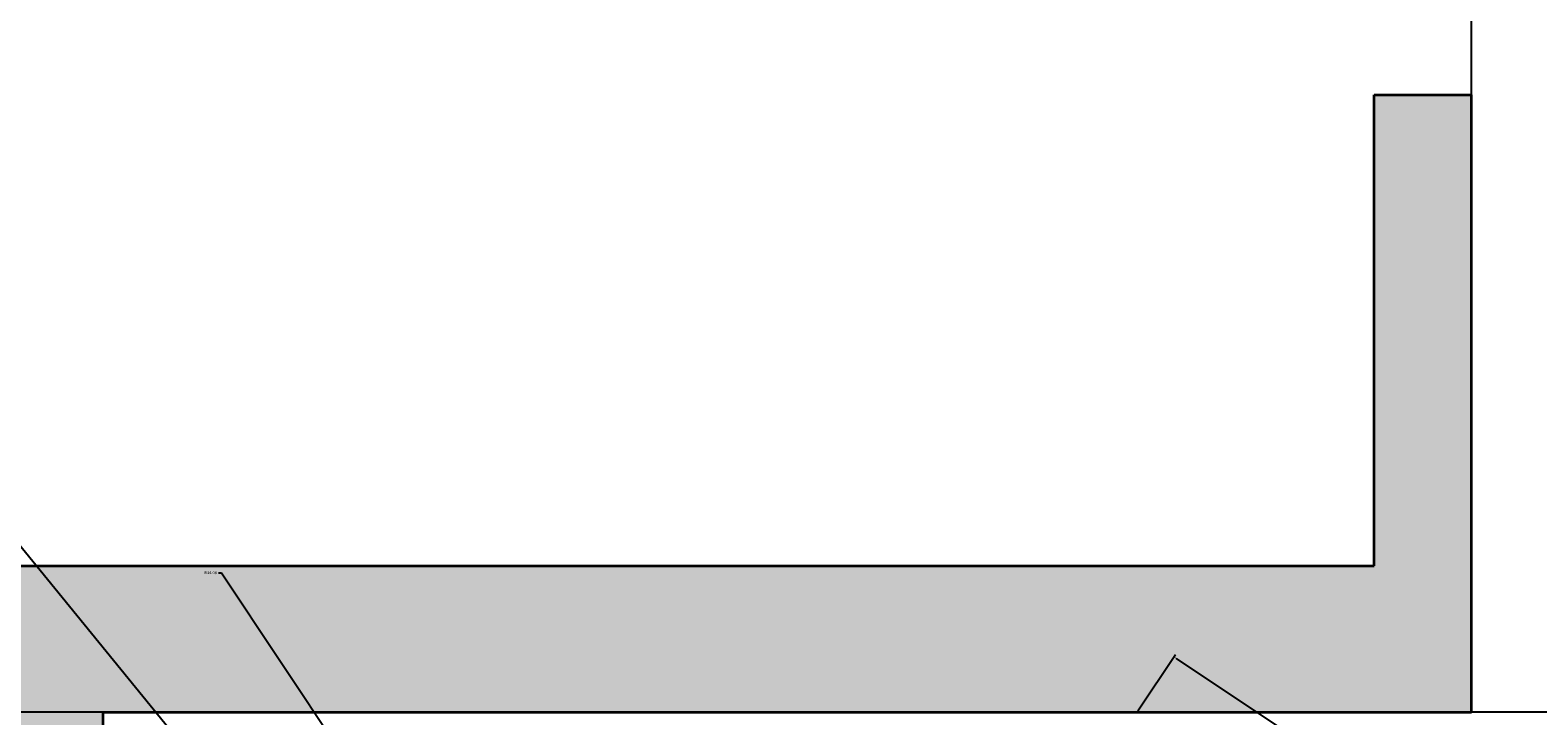
# Model space of a CAD drawing. Units: inches. Extents: x 2549 to 3108, y 1683 to 2362.
# Tile 5 of 30: x 2877 to 2970, y 1936 to 1979. Entities that reach past the tile are written whole.
import ezdxf

# ---------------------------------------------------------------- set-up
doc = ezdxf.new("R2010")
doc.units = ezdxf.units.IN
for name, color, linetype, lineweight in [('A-ANNO-DIMS', 2, 'Continuous', 18), ('A-WALL', 7, 'Continuous', 35), ('A-WALL-PATT', 89, 'Continuous', 13)]:
    doc.layers.add(name, color=color, linetype=linetype, lineweight=lineweight)
doc.layers.add('C-PKNG-VEHI-PATT', color=251, linetype='Continuous', lineweight=13, true_color=0x636466)
doc.layers.add('C-PVMT-PATT', color=9, linetype='Continuous', lineweight=13, true_color=0xc7c8ca)
doc.styles.get("Standard").update_dxf_attribs({"font": 'arial.ttf'})
doc.dimstyles.get("Standard").update_dxf_attribs({"dimtxt": 0.18, "dimasz": 0.18, "dimexe": 0.18, "dimexo": 0.0625, "dimgap": 0.09, "dimtad": 0, "dimtih": 1, "dimtoh": 1, "dimdec": 4, "dimzin": 0, "dimdsep": 46, "dimtxsty": 'Standard', "dimcen": 0.09, "dimadec": 0, "dimazin": 0, "dimtfac": 1, "dimtdec": 4, "dimtofl": 0, "dimtmove": 0, "dimatfit": 3, "dimfxl": 1, "dimtolj": 1, "dimtzin": 0, "dimarcsym": 0})

# ---------------------------------------------------------------- blocks, each defined once
blk = doc.blocks.new('*D19')
at = {"layer": 'A-ANNO-DIMS', "color": 0, "lineweight": -2, "transparency": 16777216}
for p, q in [((2945.38949374051, 1936.610352371541), (2947.701205969521, 1940.077920715058)), ((2947.751128987182, 1939.828305626757), (2957.49632815957, 1933.331506178498)), ((2967.782816554333, 1926.473847248657), (2958.037617381944, 1932.970646696915)), ((2965.720719413623, 1923.0562019228), (2968.032431642634, 1926.523770266317))]:
    blk.add_line(p, q, dxfattribs=at)
at = {"layer": 'A-ANNO-DIMS', "color": 0, "transparency": 16777216}
for points in [[(2947.767769993069, 1939.853267135587), (2947.734487981295, 1939.803344117927), (2947.6013599342, 1939.928151662078)], [(2967.799457560219, 1926.498808757487), (2967.766175548446, 1926.448885739827), (2967.932585607313, 1926.374001213336)]]:
    blk.add_solid(points, dxfattribs=at)
at = {"layer": 'Defpoints', "color": 0, "transparency": 16777216}
for p in [(2947.6013599342, 1939.928151662078), (2945.354824978246, 1936.558349228145), (2965.686050651358, 1923.004198779404)]:
    blk.add_point(p, dxfattribs=at)
at = {"layer": 'A-ANNO-DIMS', "color": 0, "transparency": 16777216, "insert": (2957.766972770757, 1933.151076437707), "char_height": 0.18, "attachment_point": 5}
blk.add_mtext('\\A1;24 TYP.', dxfattribs=at)
blk = doc.blocks.new('*D46')
at = {"layer": 'A-ANNO-DIMS', "color": 0, "lineweight": -2, "transparency": 16777216}
for p, q in [((2812.642666, 2140.461244), (2812.642666, 1683.443744)), ((3034.642666, 2134.461244), (3034.642666, 1683.443744)), ((2812.822666, 1683.623744), (2923.35320488131, 1683.623744)), ((3034.462666, 1683.623744), (2923.932127118691, 1683.623744))]:
    blk.add_line(p, q, dxfattribs=at)
at = {"layer": 'A-ANNO-DIMS', "color": 0, "transparency": 16777216}
for points in [[(2812.822666, 1683.653744), (2812.822666, 1683.593744), (2812.642666, 1683.623744)], [(3034.462666, 1683.653744), (3034.462666, 1683.593744), (3034.642666, 1683.623744)]]:
    blk.add_solid(points, dxfattribs=at)
at = {"layer": 'Defpoints', "color": 0, "transparency": 16777216}
for p in [(2812.642666, 2140.523744), (3034.642666, 2134.523744), (3034.642666, 1683.623744)]:
    blk.add_point(p, dxfattribs=at)
at = {"layer": 'A-ANNO-DIMS', "color": 0, "transparency": 16777216, "insert": (2923.642666000001, 1683.623744), "char_height": 0.18, "attachment_point": 5}
blk.add_mtext('\\A1;222', dxfattribs=at)
blk = doc.blocks.new('*D56')
at = {"layer": 'A-ANNO-DIMS', "color": 0, "lineweight": -2, "transparency": 16777216}
for p, q in [((3043.580166000001, 1936.523744000001), (2549.424763000002, 1936.523744000001)), ((2549.604763000002, 1936.343744000001), (2549.604763000002, 1911.205647137791)), ((2549.604763000002, 1885.703744000001), (2549.604763000002, 1910.841840862211)), ((3043.580166000001, 1885.523744000001), (2549.424763000002, 1885.523744000001))]:
    blk.add_line(p, q, dxfattribs=at)
at = {"layer": 'A-ANNO-DIMS', "color": 0, "transparency": 16777216}
for points in [[(2549.574763000002, 1936.343744000001), (2549.634763000002, 1936.343744000001), (2549.604763000002, 1936.523744000001)], [(2549.574763000002, 1885.703744000001), (2549.634763000002, 1885.703744000001), (2549.604763000002, 1885.523744000001)]]:
    blk.add_solid(points, dxfattribs=at)
at = {"layer": 'Defpoints', "color": 0, "transparency": 16777216}
for p in [(2549.604763000002, 1936.523744000001), (3043.642666000001, 1936.523744000001), (3043.642666000001, 1885.523744000001)]:
    blk.add_point(p, dxfattribs=at)
at = {"layer": 'A-ANNO-DIMS', "color": 0, "transparency": 16777216, "insert": (2549.604763000002, 1911.023743999999), "char_height": 0.18, "attachment_point": 5}
blk.add_mtext('\\A1;51', dxfattribs=at)
blk = doc.blocks.new('*D57')
at = {"layer": 'A-ANNO-DIMS', "color": 0, "lineweight": -2, "transparency": 16777216}
for p, q in [((2965.93514, 1936.586244), (2965.93514, 2362.322518)), ((2966.11514, 2362.142518), (2999.912081717599, 2362.142518)), ((3034.462666, 2362.142518), (3000.665724282401, 2362.142518)), ((3034.642666, 1936.586244), (3034.642666, 2362.322518))]:
    blk.add_line(p, q, dxfattribs=at)
at = {"layer": 'A-ANNO-DIMS', "color": 0, "transparency": 16777216}
for points in [[(2966.11514, 2362.172518), (2966.11514, 2362.112518), (2965.93514, 2362.142518)], [(3034.462666, 2362.172518), (3034.462666, 2362.112518), (3034.642666, 2362.142518)]]:
    blk.add_solid(points, dxfattribs=at)
at = {"layer": 'Defpoints', "color": 0, "transparency": 16777216}
for p in [(3034.642666, 2362.142518), (2965.93514, 1936.523744), (3034.642666, 1936.523744)]:
    blk.add_point(p, dxfattribs=at)
at = {"layer": 'A-ANNO-DIMS', "color": 0, "transparency": 16777216, "insert": (3000.288903, 2362.142518), "char_height": 0.18, "attachment_point": 5}
blk.add_mtext('\\A1;68.71', dxfattribs=at)
blk = doc.blocks.new('*D66')
at = {"layer": 'A-ANNO-DIMS', "color": 0, "lineweight": -2, "transparency": 16777216}
for p, q in [((2872.93362808891, 1950.941863936075), (2873.11362808891, 1950.941863936074)), ((2873.11362808891, 1950.941863936074), (2897.37882396306, 1921.218856531219)), ((2938.034368999999, 1871.308682999998), (2938.214368999999, 1871.308682999999)), ((2938.124368999999, 1871.218682999999), (2938.124369, 1871.398682999999))]:
    blk.add_line(p, q, dxfattribs=at)
at = {"layer": 'A-ANNO-DIMS', "color": 0, "transparency": 16777216}
blk.add_solid([(2897.402063218263, 1921.237828537375), (2897.355584707857, 1921.199884525062), (2897.492655999999, 1921.079420999999)], dxfattribs=at)
at = {"layer": 'Defpoints', "color": 0, "transparency": 16777216}
for p in [(2897.492655999999, 1921.079420999999), (2938.124369, 1871.308682999999)]:
    blk.add_point(p, dxfattribs=at)
at = {"layer": 'A-ANNO-DIMS', "color": 0, "transparency": 16777216, "insert": (2872.258198348119, 1950.941863936074), "char_height": 0.18, "attachment_point": 5}
blk.add_mtext('\\A1;2X R64.25', dxfattribs=at)
blk = doc.blocks.new('*D67')
at = {"layer": 'A-ANNO-DIMS', "color": 0, "lineweight": -2, "transparency": 16777216}
for p, q in [((2888.742267019754, 1945.111459470369), (2888.922267019754, 1945.111459470369)), ((2888.922267019754, 1945.111459470369), (2900.166103391877, 1928.245844671111)), ((2919.082088, 1899.737104), (2919.262088, 1899.737104)), ((2919.172088000001, 1899.647104000001), (2919.172088, 1899.827104))]:
    blk.add_line(p, q, dxfattribs=at)
at = {"layer": 'A-ANNO-DIMS', "color": 0, "transparency": 16777216}
blk.add_solid([(2900.191064837062, 1928.262485772465), (2900.141141946692, 1928.229203569756), (2900.265950000001, 1928.096076)], dxfattribs=at)
at = {"layer": 'Defpoints', "color": 0, "transparency": 16777216}
for p in [(2900.265950000001, 1928.096076), (2919.172088, 1899.737104)]:
    blk.add_point(p, dxfattribs=at)
at = {"layer": 'A-ANNO-DIMS', "color": 0, "transparency": 16777216, "insert": (2888.262246555907, 1945.111459470368), "char_height": 0.18, "attachment_point": 5}
blk.add_mtext('\\A1;R34.08', dxfattribs=at)

msp = doc.modelspace()

# ---------------------------------------------------------------- hatches: boundary and pattern name
at = {"layer": 'A-WALL-PATT'}
h = msp.add_hatch(color=256, dxfattribs=at)
h.dxf.hatch_style = 1
h.paths.add_polyline_path([(2638.642666391656, 2272.523744486262), (3034.642666391656, 2272.523744486262), (3034.642666391656, 1936.523744486262), (3043.642666391656, 1936.523744486262), (3043.642666391656, 2281.523744486262), (2629.642666391656, 2281.523744486262), (2629.642666391656, 2074.523744486262), (2812.642666391655, 2074.523744486262), (2812.642666391655, 2140.523744486262), (2785.717675498527, 2140.523744486262), (2785.717675498527, 2134.523744486262), (2806.642666391656, 2134.523744486262), (2806.642666391656, 2080.523744486262), (2638.642666391656, 2080.523744486262)])
h.paths.add_polyline_path([(2638.642666391656, 1972.523744486262), (2662.642666391656, 1972.523744486262), (2662.642666391656, 2041.055679691546), (2653.642666391655, 2041.055679691546), (2653.642666391656, 1978.523744486262), (2629.642666391656, 1978.523744486262), (2629.642666391656, 1795.523744486262), (2662.642666391656, 1795.523744486262), (2881.642666391656, 1795.523744486262), (2881.642666391656, 1936.523744486262), (2965.935139880862, 1936.523744486262), (2965.935139880862, 1974.543933838007), (2959.935139880861, 1974.543933838007), (2959.935139880861, 1945.523744486262), (2881.642666391656, 1945.523744486262), (2872.642666391655, 1945.523744486262), (2872.642666391655, 1804.523744486262), (2662.642666391656, 1804.523744486262), (2638.642666391656, 1804.523744486262)])
at = {"layer": 'C-PKNG-VEHI-PATT'}
h = msp.add_hatch(color=256, dxfattribs=at)
h.dxf.hatch_style = 1
edge = h.paths.add_edge_path()
edge.add_ellipse((2935.725796552836, 1791.96404850691), major_axis=(-50.6600031146233, 6.78e-13), ratio=0.8423038695439883, start_angle=248.1650462032912, end_angle=265.7225790369452)
edge.add_line((2938.911028887629, 1834.550737322417), (2925.865275339109, 1834.550737322417))
edge.add_ellipse((2929.050507673901, 1791.964048506909), major_axis=(50.66000311462998, 7.2698e-12), ratio=0.8423038695438956, start_angle=94.27742096304536, end_angle=111.8349537966996)
edge.add_line((2912.850791291541, 1832.394679033669), (2914.204376096751, 1822.249450253823))
edge.add_ellipse((2930.653832861207, 1783.102276333115), major_axis=(-49.30143828149606, 1.1087e-12), ratio=0.8423038695440098, start_angle=-85.12993040286318, end_angle=-67.20808512241217, ccw=False)
edge.add_line((2927.124659327709, 1824.522535937876), (2937.65164489903, 1824.522535937876))
edge.add_ellipse((2934.122471365533, 1783.102276333124), major_axis=(49.30143828148681, 7.803e-13), ratio=0.8423038695439693, start_angle=67.20808512240922, end_angle=85.12993040286312, ccw=False)
edge.add_line((2950.571928129987, 1822.249450253823), (2951.925512935197, 1832.394679033669))
edge = h.paths.add_edge_path()
edge.add_ellipse((2903.479330909537, 1857.335124490177), major_axis=(-34.79790434319148, 3.2087e-12), ratio=0.8423038695440206, start_angle=180.0000000000052, end_angle=209.4385695979841)
edge.add_ellipse((2961.296973317201, 1857.335124490177), major_axis=(34.79790434319149, 1.2616e-12), ratio=0.8423038695439669, start_angle=150.5614304020187, end_angle=179.9999999999979)
edge.add_line((2926.49906897401, 1857.335124490177), (2926.49906897401, 1843.76085484809))
edge.add_ellipse((2924.125124210826, 1844.314306179491), major_axis=(-0.2209272451118966, 3.927824345135514), ratio=0.6038335755719296, start_angle=89.00201427502537, end_angle=253.65740804569998, ccw=False)
edge.add_line((2921.751179447642, 1844.222223668088), (2921.751179447642, 1853.39746861696))
edge.add_line((2921.751179447642, 1853.39746861696), (2925.26903797625, 1855.848425453852))
edge.add_ellipse((2925.478177919096, 1855.493055533625), major_axis=(0.4583993962922678, 2.303e-12), ratio=0.8423038695418179, start_angle=89.9999999997122, end_angle=134.4802108822853, ccw=False)
edge.add_line((2925.478177919095, 1855.879167118917), (2926.49906897401, 1855.879167118917))
edge.add_line((2926.49906897401, 1855.879167118917), (2926.49906897401, 1857.335124490177))
edge.add_ellipse((2961.296973317201, 1857.335124490177), major_axis=(34.79790434319149, 1.2616e-12), ratio=0.8423038695439669, start_angle=150.5614304020187, end_angle=179.999999999998, ccw=False)
edge.add_line((2932.388152113369, 1873.650056952746), (2932.388152113369, 1875.780055063896))
edge.add_ellipse((2932.388152113369, 1875.393943478604), major_axis=(0.4583993962904624, 1e-16), ratio=0.8423038695446395, start_angle=89.99999999999999, end_angle=127.9331304598429)
edge.add_line((2932.136581844764, 1875.716714504374), (2928.591534983032, 1873.756406364807))
edge.add_ellipse((2899.927094610101, 2002.469218934773), major_axis=(155.4756451483881, 9.82606e-11), ratio=0.842303869543439, start_angle=-80.74343399283458, end_angle=-77.44506735589891, ccw=False)
edge.add_ellipse((2949.440169726089, 1715.215149574257), major_axis=(-189.1421864819335, 9.35831e-11), ratio=0.8423038695443681, start_angle=-79.79046100282835, end_angle=-77.55537270652765)
edge.add_ellipse((3300.361430890526, 1852.564199885104), major_axis=(-386.1662101011402, 3.282e-12), ratio=0.8423038695438535, start_angle=-2.863714607837213, end_angle=2.198540565955553)
edge.add_ellipse((2929.050507673902, 1792.515918881865), major_axis=(-55.61920468847034, 9.624e-12), ratio=0.842303869544118, start_angle=-85.91758930883981, end_angle=-72.28004677724027, ccw=False)
edge.add_line((2925.712863234435, 1839.27976237288), (2939.063440992303, 1839.27976237288))
edge.add_ellipse((2935.725796552836, 1792.515918881865), major_axis=(55.61920468846977, 1.19088e-11), ratio=0.8423038695441256, start_angle=72.28004677723749, end_angle=85.91758930883759, ccw=False)
edge.add_ellipse((2564.414873336211, 1852.564199885105), major_axis=(-386.166210101141, 7.3121e-12), ratio=0.8423038695442235, start_angle=177.8014594340458, end_angle=182.8637146078386)
edge.add_ellipse((2915.336134500645, 1715.215149574254), major_axis=(189.1421864814668, 5.425418e-10), ratio=0.8423038695464061, start_angle=77.5553727063904, end_angle=79.79046100269107)
edge.add_ellipse((2964.849209616638, 2002.469218934773), major_axis=(-155.4756451483861, 9.70869e-11), ratio=0.8423038695434499, start_angle=77.44506735589852, end_angle=80.74343399283418, ccw=False)
edge.add_line((2936.184769243706, 1873.756406364807), (2932.639722381973, 1875.716714504375))
edge.add_ellipse((2932.388152113369, 1875.393943478604), major_axis=(0.4583993962904624, 1e-16), ratio=0.8423038695446395, start_angle=52.06686954015704, end_angle=89.99999999999999)
edge.add_line((2932.388152113369, 1875.780055063896), (2932.388152113369, 1873.650056952746))
edge.add_ellipse((2903.479330909537, 1857.335124490177), major_axis=(-34.79790434319148, 3.2087e-12), ratio=0.8423038695440206, start_angle=180.0000000000053, end_angle=209.4385695979841, ccw=False)
edge.add_line((2938.277235252728, 1857.335124490177), (2938.277235252728, 1855.879167118917))
edge.add_line((2938.277235252728, 1855.879167118917), (2939.405880844674, 1855.879167118917))
edge.add_ellipse((2939.298126307642, 1855.493055533625), major_axis=(-0.4583993962922676, 2.3028e-12), ratio=0.8423038695418185, start_angle=225.5197891177147, end_angle=270.00000000028786, ccw=False)
edge.add_line((2939.590297193029, 1855.790576266728), (2943.025124779096, 1853.39746861696))
edge.add_line((2943.025124779096, 1853.39746861696), (2943.025124779096, 1844.222223668088))
edge.add_ellipse((2940.651180015912, 1844.314306179491), major_axis=(0.2209272451118966, 3.927824345135514), ratio=0.6038335755719296, start_angle=106.3425919543001, end_angle=270.9979857249746, ccw=False)
edge.add_line((2938.277235252728, 1843.76085484809), (2938.277235252728, 1857.335124490177))
edge = h.paths.add_edge_path()
edge.add_ellipse((2932.388152113369, 1865.19731394932), major_axis=(91.08099646002908, 7.134e-13), ratio=0.8423038695439837, start_angle=256.4018653097688, end_angle=283.5981346902299, ccw=False)
edge.add_line((2914.204376096751, 1790.023884530285), (2914.204376096751, 1778.36217788565))
edge.add_ellipse((2932.388152113369, 1853.535607304685), major_axis=(91.08099646002908, 7.134e-13), ratio=0.8423038695439837, start_angle=256.4018653097688, end_angle=283.5981346902299)
edge.add_line((2950.571928129987, 1778.36217788565), (2950.571928129987, 1790.023884530285))
edge = h.paths.add_edge_path()
edge.add_ellipse((2948.738330544823, 1772.31452600415), major_axis=(1.833597585163715, 1.1861e-12), ratio=0.8423038695440299, start_angle=-3.70558e-11, end_angle=89.99999999996297)
edge.add_line((2948.738330544824, 1773.85897234532), (2916.037973681915, 1773.858972345321))
edge.add_ellipse((2916.037973681915, 1772.314526004151), major_axis=(1.833597585163716, 6.788e-13), ratio=0.84230386954403, start_angle=89.9999999999788, end_angle=179.9999999999787)
edge.add_line((2914.204376096751, 1772.314526004151), (2914.204376096751, 1760.255799913309))
edge.add_line((2914.204376096751, 1760.255799913309), (2950.571928129987, 1760.255799913308))
edge.add_line((2950.571928129987, 1760.255799913308), (2950.571928129987, 1772.31452600415))
h.paths.add_polyline_path([(2748.849609196547, 2101.638310911291), (2798.147998217048, 2101.638310911291), (2798.147998217048, 2111.424826549233), (2748.849609196547, 2111.424826549233)], flags=9)
h.paths.add_polyline_path([(2685.208067619545, 2101.488974631509), (2719.325307162104, 2101.488974631509), (2719.325307162104, 2111.281945754699), (2685.208067619545, 2111.281945754699)], flags=9)
h.paths.add_polyline_path([(2814.685179139321, 1907.132804880864), (2847.838399551318, 1907.132804880864), (2847.838399551318, 1916.925776004054), (2814.685179139321, 1916.925776004054)], flags=9)
h.paths.add_polyline_path([(2814.390575309562, 1835.586397562281), (2848.017197973174, 1835.586397562281), (2848.017197973174, 1845.379368685471), (2814.390575309562, 1845.379368685471)], flags=9)
h.paths.add_polyline_path([(2800.524456569608, 1759.167447237475), (2853.743476964851, 1759.167447237475), (2853.743476964851, 1768.953962875417), (2800.524456569608, 1768.953962875417)], flags=9)
h.paths.add_polyline_path([(2972.461062245805, 1807.33049128039), (3015.394342810494, 1807.33049128039), (3015.394342810494, 1817.117006918332), (2972.461062245805, 1817.117006918332)], flags=9)
h.paths.add_polyline_path([(2902.332650472062, 1888.673085326325), (2937.913133337796, 1888.673085326325), (2937.913133337796, 1898.466056449515), (2902.332650472062, 1898.466056449515)], flags=9)
h.paths.add_polyline_path([(2712.17793111998, 1878.903902566108), (2754.125674269943, 1878.903902566108), (2754.125674269943, 1888.69041820405), (2712.17793111998, 1888.69041820405)], flags=9)
h.paths.add_polyline_path([(2614.005606808349, 2012.811964980989), (2650.025062671036, 2012.811964980989), (2650.025062671036, 2022.437093487698), (2614.005606808349, 2022.437093487698)], flags=9)
h.paths.add_polyline_path([(2713.312922761346, 2003.164487508756), (2747.423706818656, 2003.164487508756), (2747.423706818656, 2012.951003146698), (2713.312922761346, 2012.951003146698)], flags=9)
h.paths.add_polyline_path([(2950.137937233872, 2001.693439459313), (2982.299164745893, 2001.693439459313), (2982.299164745893, 2011.479955097255), (2950.137937233872, 2011.479955097255)], flags=9)
h.paths.add_polyline_path([(2940.863994744806, 2238.553674899427), (2997.506574150595, 2238.553674899427), (2997.506574150595, 2248.346646022617), (2940.863994744806, 2248.346646022617)], flags=9)
h.paths.add_polyline_path([(2821.545730132573, 2202.834824551463), (2855.662969675132, 2202.834824551463), (2855.662969675132, 2212.627795674654), (2821.545730132573, 2212.627795674654)], flags=9)
h.paths.add_polyline_path([(2661.802564922812, 2238.624912952816), (2718.445144328601, 2238.624912952816), (2718.445144328601, 2248.417884076006), (2661.802564922812, 2248.417884076006)], flags=9)
at = {"layer": 'C-PVMT-PATT'}
h = msp.add_hatch(color=256, dxfattribs=at)
h.dxf.hatch_style = 1
h.paths.add_polyline_path([(3067.642666391656, 2305.523744486262), (2605.642666391656, 2305.523744486262), (2605.642666391656, 2074.523744486262), (2629.642666391656, 2074.523744486262), (2629.642666391656, 2281.523744486262), (3043.642666391656, 2281.523744486262), (3043.642666391656, 1885.523744486263), (3043.642666391656, 1872.874514030248), (3031.167181590035, 1872.874514030248), (3031.167181590035, 1862.573058982011), (2995.805391311171, 1862.573058982011), (2995.805391311171, 1872.874514030248), (2983.175155144805, 1872.874514030248), (2983.175155144805, 1885.523744486262), (2881.642666391656, 1885.523744486263), (2881.642666391656, 1795.523744486262), (2751.09773888662, 1795.523744486262), (2751.09773888662, 1761.523744486262), (2786.157685455576, 1761.523744486262), (2786.157685455577, 1723.523744486262), (2881.839988255281, 1723.523744486262), (2881.839988255281, 1714.523744486262), (3067.642666391656, 1714.523744486262), (3067.642666391656, 1723.523744486262)])
edge = h.paths.add_edge_path(flags=16)
edge.add_ellipse((2949.440169726093, 1710.96831784248), major_axis=(-194.1013880556022, 3.100242e-10), ratio=0.8423038695451509, start_angle=-77.87403444762441, end_angle=-76.21947101041059, ccw=False)
edge.add_ellipse((2949.440169726089, 1715.215149574257), major_axis=(-189.1421864819335, 9.35831e-11), ratio=0.8423038695443681, start_angle=-79.7904610028283, end_angle=-77.55537270652758, ccw=False)
edge.add_ellipse((2899.927094610101, 2002.469218934773), major_axis=(155.4756451483881, 9.82606e-11), ratio=0.842303869543439, start_angle=-80.74343399283462, end_angle=-77.44506735589897)
edge.add_line((2928.591534983032, 1873.756406364807), (2932.388152113369, 1875.855825569603))
edge.add_line((2932.388152113369, 1875.855825569603), (2936.184769243706, 1873.756406364807))
edge.add_ellipse((2964.849209616638, 2002.469218934773), major_axis=(-155.4756451483861, 9.70869e-11), ratio=0.8423038695434499, start_angle=77.4450673558985, end_angle=80.74343399283416)
edge.add_ellipse((2915.336134500645, 1715.215149574254), major_axis=(189.1421864814668, 5.425418e-10), ratio=0.8423038695464061, start_angle=77.55537270639041, end_angle=79.79046100269102, ccw=False)
edge.add_ellipse((2915.336134500645, 1710.96831784248), major_axis=(-194.1013880561466, 2.794238e-10), ratio=0.8423038695428703, start_angle=256.2194710105847, end_angle=257.8740344477983, ccw=False)
edge.add_ellipse((2628.287132012546, 1850.261185811051), major_axis=(-327.2531525161749, 1.24457e-11), ratio=0.8423038695440036, start_angle=182.1799503136474, end_angle=183.6504275857012, ccw=False)
edge.add_ellipse((2955.563661936079, 1861.933375066942), major_axis=(-0.9167987925820851, 6.203e-13), ratio=0.8423038695438211, start_angle=180.0000000000388, end_angle=270.00000000003877, ccw=False)
edge.add_line((2956.480460728661, 1862.385732927092), (2956.480460728661, 1846.486613953928))
edge.add_ellipse((2955.563661936079, 1846.938971814078), major_axis=(-0.9167987925816303, 6.983e-13), ratio=0.8423038695442389, start_angle=90.0000000000436, end_angle=180.0000000000437, ccw=False)
edge.add_ellipse((-3607.060581297885, 1835.831972437108), major_axis=(-6562.624243233964, 2.000376e-10), ratio=0.8423038695434055, start_angle=179.6161332212093, end_angle=180.0902290885961, ccw=False)
edge.add_ellipse((2955.563661936079, 1791.092611498023), major_axis=(0.9167987925816303, 1.8053e-12), ratio=0.8423038695442389, start_angle=-1.127773430198431e-10, end_angle=89.99999999988711, ccw=False)
edge.add_line((2956.480460728661, 1791.544969358173), (2956.480460728661, 1775.645850385008))
edge.add_ellipse((2955.563661936079, 1776.098208245159), major_axis=(0.9167987925816303, 5.91e-14), ratio=0.8423038695442391, start_angle=269.9999999999963, end_angle=359.9999999999963, ccw=False)
edge.add_ellipse((-3607.060581297885, 1835.831972437108), major_axis=(-6562.624243233964, 2.000376e-10), ratio=0.8423038695434055, start_angle=179.3813568036826, end_angle=179.4717285281838, ccw=False)
edge.add_ellipse((2954.590723441648, 1763.876816393945), major_axis=(-1.375198188872997, 3.586e-13), ratio=0.8423038695436877, start_angle=179.3717627838213, end_angle=248.4647566010281, ccw=False)
edge.add_ellipse((-3607.518980694323, 1835.831972435604), major_axis=(-6564.040927375597, 4.0829067806e-06), ratio=0.8423038626957529, start_angle=179.3534459385899, end_angle=179.371762819423, ccw=False)
edge.add_ellipse((2952.682914207262, 1761.800246254478), major_axis=(3.250281735962, 3.921e-13), ratio=0.8423038695438826, start_angle=-89.99999999994031, end_angle=-0.6465540970884831, ccw=False)
edge.add_line((2952.682914207266, 1759.06252137117), (2912.093390019471, 1759.062521371171))
edge.add_ellipse((2912.093390019478, 1761.800246254481), major_axis=(3.250281735963338, 1.2841e-12), ratio=0.8423038695440954, start_angle=180.6465540970387, end_angle=269.99999999984414, ccw=False)
edge.add_ellipse((9472.295284948175, 1835.831972439052), major_axis=(-6564.040927413921, 8.323842912e-07), ratio=0.8423038709559154, start_angle=0.6282372235086768, end_angle=0.646554104341817, ccw=False)
edge.add_ellipse((2910.185580785089, 1763.876816393947), major_axis=(1.375198188873441, 9.687e-13), ratio=0.8423038695438604, start_angle=111.53524350397811, end_angle=180.6282372161342, ccw=False)
edge.add_ellipse((9471.836885542962, 1835.831972437208), major_axis=(-6562.624243252301, 3.836442e-10), ratio=0.8423038695462286, start_angle=0.5282714718206876, end_angle=0.6465540970643247, ccw=False)
edge.add_ellipse((2909.212642290659, 1776.098208245159), major_axis=(-0.9167987925820851, 6.203e-13), ratio=0.8423038695438211, start_angle=3.8824055081931874e-11, end_angle=90.00000000003882, ccw=False)
edge.add_line((2908.295843498077, 1775.645850385009), (2908.295843498077, 1791.544969358173))
edge.add_ellipse((2909.212642290659, 1791.092611498023), major_axis=(-0.9167987925820851, 4.868e-13), ratio=0.8423038695438213, start_angle=-89.99999999996948, end_angle=3.041122909053229e-11, ccw=False)
edge.add_ellipse((9471.836885542962, 1835.831972437208), major_axis=(-6562.624243252301, 3.836442e-10), ratio=0.8423038695462286, start_angle=-0.09022908858980827, end_angle=0.38386677879560693, ccw=False)
edge.add_ellipse((2909.212642290658, 1846.938971814078), major_axis=(-0.9167987925816306, 1.1661e-12), ratio=0.8423038695442389, start_angle=7.287326297955588e-11, end_angle=90.00000000007287, ccw=False)
edge.add_line((2908.295843498077, 1846.486613953928), (2908.295843498077, 1862.385732927092))
edge.add_ellipse((2909.212642290658, 1861.933375066942), major_axis=(0.9167987925816303, 1.1659e-12), ratio=0.8423038695442391, start_angle=89.99999999992713, end_angle=179.9999999999272, ccw=False)
edge.add_ellipse((3236.489172214191, 1850.261185811051), major_axis=(327.2531525161745, 3.33005e-11), ratio=0.8423038695444386, start_angle=176.3495724142951, end_angle=177.820049686349, ccw=False)
edge = h.paths.add_edge_path(flags=0)
edge.add_ellipse((2903.479330909537, 1857.335124490177), major_axis=(-34.79790434319148, 3.2087e-12), ratio=0.8423038695440206, start_angle=180.0000000000053, end_angle=209.4385695979841, ccw=False)
edge.add_line((2938.277235252728, 1857.335124490177), (2938.277235252728, 1855.879167118917))
edge.add_line((2938.277235252728, 1855.879167118917), (2939.463142736354, 1855.879167118917))
edge.add_line((2939.463142736354, 1855.879167118917), (2943.025124779096, 1853.39746861696))
edge.add_line((2943.025124779096, 1853.39746861696), (2943.025124779096, 1844.222223668088))
edge.add_ellipse((2940.651180015912, 1844.314306179491), major_axis=(0.2209272451118966, 3.927824345135514), ratio=0.6038335755719296, start_angle=106.3425919543001, end_angle=270.9979857249746, ccw=False)
edge.add_line((2938.277235252728, 1843.76085484809), (2938.277235252728, 1857.335124490177))
edge.add_ellipse((2903.479330909537, 1857.335124490177), major_axis=(-34.79790434319148, 3.2087e-12), ratio=0.8423038695440206, start_angle=180.0000000000052, end_angle=209.4385695979841)
edge.add_ellipse((2961.296973317201, 1857.335124490177), major_axis=(34.79790434319149, 1.2616e-12), ratio=0.8423038695439669, start_angle=150.5614304020187, end_angle=179.9999999999979)
edge.add_line((2926.49906897401, 1857.335124490177), (2926.49906897401, 1843.76085484809))
edge.add_ellipse((2924.125124210826, 1844.314306179491), major_axis=(-0.2209272451118966, 3.927824345135514), ratio=0.6038335755719296, start_angle=89.00201427502537, end_angle=253.65740804569998, ccw=False)
edge.add_line((2921.751179447642, 1844.222223668088), (2921.751179447642, 1853.39746861696))
edge.add_line((2921.751179447642, 1853.39746861696), (2925.313161490385, 1855.879167118917))
edge.add_line((2925.313161490385, 1855.879167118917), (2926.49906897401, 1855.879167118917))
edge.add_line((2926.49906897401, 1855.879167118917), (2926.49906897401, 1857.335124490177))
edge.add_ellipse((2961.296973317201, 1857.335124490177), major_axis=(34.79790434319149, 1.2616e-12), ratio=0.8423038695439669, start_angle=150.5614304020187, end_angle=179.999999999998, ccw=False)
edge = h.paths.add_edge_path(flags=0)
edge.add_ellipse((2929.050507673901, 1791.964048506909), major_axis=(50.66000311462998, 7.2698e-12), ratio=0.8423038695438956, start_angle=94.2774209630453, end_angle=111.8349537966997, ccw=False)
edge.add_line((2925.865275339109, 1834.550737322417), (2938.911028887629, 1834.550737322417))
edge.add_ellipse((2935.725796552836, 1791.96404850691), major_axis=(-50.6600031146233, 6.78e-13), ratio=0.8423038695439883, start_angle=248.16504620329118, end_angle=265.72257903694526, ccw=False)
edge.add_line((2951.925512935197, 1832.394679033669), (2950.571928129987, 1822.249450253823))
edge.add_ellipse((2934.122471365533, 1783.102276333124), major_axis=(49.30143828148681, 7.803e-13), ratio=0.8423038695439693, start_angle=67.20808512240917, end_angle=85.12993040286312)
edge.add_line((2937.651644899029, 1824.522535937876), (2927.12465932771, 1824.522535937876))
edge.add_ellipse((2930.653832861207, 1783.102276333115), major_axis=(-49.30143828149606, 1.1087e-12), ratio=0.8423038695440098, start_angle=-85.12993040286322, end_angle=-67.20808512241221)
edge.add_line((2914.204376096751, 1822.249450253823), (2912.850791291541, 1832.394679033669))
edge = h.paths.add_edge_path(flags=0)
edge.add_line((2910.133794844343, 1829.46512489105), (2912.643202843121, 1821.271117801794))
edge.add_ellipse((5203.77865552976, 1816.436683891122), major_axis=(-2291.142641748503, 9.8835e-11), ratio=0.8423038695495838, start_angle=-0.1208973690305054, end_angle=0.3640763488925343)
edge.add_line((2912.701209242743, 1801.878223466977), (2910.33046059899, 1792.569831244782))
edge.add_ellipse((9471.836885542954, 1835.831972437156), major_axis=(-6561.70744445971, 7.61654e-11), ratio=0.8423038695443023, start_angle=0.055594313499796044, end_angle=0.37776419391019544, ccw=False)
edge = h.paths.add_edge_path(flags=0)
edge.add_ellipse((-3607.060581316224, 1835.831972437187), major_axis=(6561.707444459722, 1.43187e-10), ratio=0.8423038695443235, start_angle=-0.37776419391110494, end_angle=-0.05559431350059185, ccw=False)
edge.add_line((2954.445843627751, 1792.569831244769), (2952.075094983995, 1801.878223466976))
edge.add_ellipse((660.9976486969767, 1816.436683891133), major_axis=(2291.142641748505, 5.276994e-10), ratio=0.842303869552366, start_angle=-0.3640763489035208, end_angle=0.1208973690194708)
edge.add_line((2952.133101383619, 1821.2711178018), (2954.642509382395, 1829.46512489105))
edge = h.paths.add_edge_path(flags=0)
edge.add_ellipse((2932.388152113369, 1865.19731394932), major_axis=(91.08099646002908, 7.134e-13), ratio=0.8423038695439837, start_angle=256.4018653097688, end_angle=283.5981346902299)
edge.add_line((2950.571928129987, 1790.023884530285), (2950.571928129987, 1778.362177885651))
edge.add_ellipse((2932.388152113369, 1853.535607304685), major_axis=(91.08099646002908, 7.134e-13), ratio=0.8423038695439837, start_angle=256.4018653097688, end_angle=283.5981346902299, ccw=False)
edge.add_line((2914.204376096751, 1778.362177885651), (2914.204376096751, 1790.023884530285))
edge = h.paths.add_edge_path(flags=0)
edge.add_line((2916.037973681915, 1773.858972345321), (2948.738330544823, 1773.85897234532))
edge.add_ellipse((2948.738330544823, 1772.31452600415), major_axis=(1.833597585163715, 1.1861e-12), ratio=0.8423038695440299, start_angle=-3.7118752516107634e-11, end_angle=89.999999999963, ccw=False)
edge.add_line((2950.571928129987, 1772.31452600415), (2950.571928129987, 1760.255799913308))
edge.add_line((2950.571928129987, 1760.255799913308), (2914.204376096751, 1760.255799913309))
edge.add_line((2914.204376096751, 1760.255799913309), (2914.204376096751, 1772.314526004151))
edge.add_ellipse((2916.037973681915, 1772.314526004151), major_axis=(1.833597585163716, 6.788e-13), ratio=0.84230386954403, start_angle=89.9999999999788, end_angle=179.9999999999788, ccw=False)
h.paths.add_polyline_path([(2629.642666391656, 1978.523744486262), (2605.642666391656, 1978.523744486262), (2605.642666391656, 1723.523744486262), (2629.642666391656, 1723.523744486262), (2629.642666391656, 1795.523744486262)], flags=17)
h.paths.add_polyline_path([(2800.524456569608, 1759.167447237475), (2853.743476964851, 1759.167447237475), (2853.743476964851, 1768.953962875417), (2800.524456569608, 1768.953962875417)], flags=24)
h.paths.add_polyline_path([(2972.461062245805, 1807.33049128039), (3015.394342810494, 1807.33049128039), (3015.394342810494, 1817.117006918332), (2972.461062245805, 1817.117006918332)], flags=24)

# ---------------------------------------------------------------- linework, layer by layer
at = {"layer": 'A-WALL'}
for p, q in [((2959.935139880861, 1945.523744486262), (2959.935139880861, 1974.543933838007)), ((2959.935139880861, 1974.543933838007), (2965.935139880862, 1974.543933838007)), ((2965.935139880862, 1936.523744486262), (2965.935139880862, 1974.543933838007)), ((2881.642666391656, 1945.523744486262), (2959.935139880861, 1945.523744486262)), ((2881.642666391656, 1795.523744486262), (2881.642666391656, 1936.523744486262)), ((2881.642666391656, 1936.523744486262), (2965.935139880862, 1936.523744486262))]:
    msp.add_line(p, q, dxfattribs=at)
msp.add_lwpolyline([(2872.642666391655, 1945.523744486262), (2881.642666391656, 1945.523744486262)], dxfattribs=at)

# ---------------------------------------------------------------- dimensions: what is measured, and where the dimension line sits
at = {"layer": 'A-ANNO-DIMS'}
for base, p1, p2, override, picture, middle in [((3034.642666, 2362.142518), (2965.93514, 1936.523744), (3034.642666, 1936.523744), {"dimdec": 2, "dimlfac": 1, "dimrnd": 0, "dimzin": 0, "dimdsep": 46, "dimlunit": 2}, '*D57', (3000.288903, 2362.142518)), ((3034.642666, 1683.623744), (2812.642666, 2140.523744), (3034.642666, 2134.523744), {"dimdec": 0, "dimlfac": 1, "dimrnd": 0, "dimzin": 0, "dimdsep": 46, "dimlunit": 2}, '*D46', (2923.642666000001, 1683.623744))]:
    dim = msp.add_linear_dim(base=base, p1=p1, p2=p2, dimstyle='Standard', override=override, dxfattribs=at)
    dim.commit()
    dim.dimension.update_dxf_attribs({"geometry": picture, "text_midpoint": middle})
dim = msp.add_radius_dim(center=(2938.124369, 1871.308682999999), mpoint=(2897.492655999999, 1921.079420999999), text='2X <>', dimstyle='Standard', override={"dimdec": 2, "dimlfac": 1, "dimrnd": 0, "dimzin": 0, "dimdsep": 46, "dimlunit": 2}, dxfattribs=at)
dim.commit()
dim.dimension.update_dxf_attribs({"geometry": '*D66', "text_midpoint": (2872.258198348119, 1950.941863936074), "dimtype": 164})
dim = msp.add_radius_dim(center=(2919.172088, 1899.737104), mpoint=(2900.265950000001, 1928.096076), dimstyle='Standard', override={"dimdec": 2, "dimlfac": 1, "dimrnd": 0, "dimzin": 0, "dimdsep": 46, "dimlunit": 2}, dxfattribs=at)
dim.commit()
dim.dimension.update_dxf_attribs({"geometry": '*D67', "text_midpoint": (2888.262246555907, 1945.111459470368), "dimtype": 164})
dim = msp.add_linear_dim(base=(2947.6013599342, 1939.928151662078), p1=(2965.686050651358, 1923.004198779404), p2=(2945.354824978246, 1936.558349228145), angle=146.3099324740215, text='<> TYP.', dimstyle='Standard', override={"dimdec": 0, "dimlfac": 1, "dimrnd": 0, "dimzin": 0, "dimdsep": 46, "dimlunit": 2}, dxfattribs=at)
dim.commit()
dim.dimension.update_dxf_attribs({"geometry": '*D19', "text_midpoint": (2957.766972770757, 1933.151076437707)})
dim = msp.add_linear_dim(base=(2549.604763000002, 1936.523744000001), p1=(3043.642666, 1885.523744), p2=(3043.642666, 1936.523744), angle=90, dimstyle='Standard', override={"dimdec": 0, "dimlfac": 1, "dimrnd": 0, "dimzin": 0, "dimdsep": 46, "dimlunit": 2}, dxfattribs=at)
dim.commit()
dim.dimension.update_dxf_attribs({"geometry": '*D56', "text_midpoint": (2549.604763000002, 1911.023743999999)})

doc.saveas('drawing.dxf')
